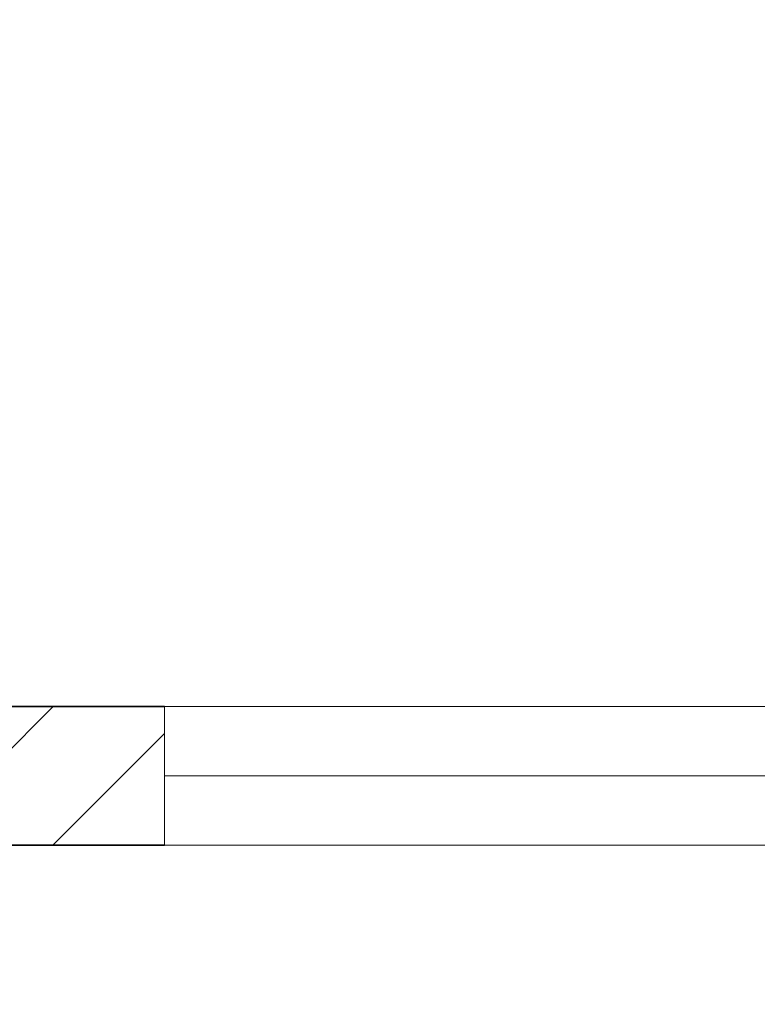
# Model space of a CAD drawing. Units: inches. Extents: x 1885 to 2748, y 783 to 2421.
# Tile 5 of 117: x 1993 to 2017, y 1082 to 1114. Entities that reach past the tile are written whole.
import ezdxf

# ---------------------------------------------------------------- set-up
doc = ezdxf.new("R2010")
doc.units = ezdxf.units.IN
doc.layers.add('A-GLAZ', color=181, linetype='Continuous', lineweight=18)
doc.layers.add('A-WALL', color=7, linetype='Continuous', lineweight=35)
doc.layers.add('A-WALL-PATT', color=85, linetype='Continuous', lineweight=13, true_color=0x58ba48)

# ---------------------------------------------------------------- blocks, each defined once
blk = doc.blocks.new('WIN-60')
for p, q in [((0.004, 59.998), (0.004, -0.002)), ((2.254, 59.998), (2.254, -0.002)), ((4.504, -0.002), (4.504, 59.998)), ((2.254, -0.002), (0.004, -0.002)), ((0.004, -0.002), (4.504, -0.002))]:
    blk.add_line(p, q)

msp = doc.modelspace()

# ---------------------------------------------------------------- hatches: boundary and pattern name
at = {"layer": 'A-WALL-PATT'}
h = msp.add_hatch(dxfattribs=at)
h.set_pattern_fill('ANSI32', color=256)
h.paths.add_polyline_path([(2007.772, 2318.006), (1980.774, 2318.006), (1980.774, 2281.215), (1985.274, 2281.215), (1985.274, 2313.506), (2007.772, 2313.506), (2007.772, 2315.756)])
h.paths.add_polyline_path([(2094.324, 2318.006), (2067.772, 2318.006), (2067.772, 2313.506), (2094.324, 2313.506), (2094.324, 2315.756)])
h.paths.add_polyline_path([(2131.367, 2315.756), (2131.367, 2318.006), (2131.189, 2318.006), (2112.609, 2318.006), (2112.609, 2313.506), (2117.274, 2313.506), (2117.274, 2255.201), (2121.774, 2255.201), (2121.774, 2313.506), (2131.367, 2313.506)])
h.paths.add_polyline_path([(2190.512, 2318.006), (2155.367, 2318.006), (2155.367, 2313.506), (2169.774, 2313.506), (2169.774, 2229.506), (2121.774, 2229.506), (2121.774, 2233.451), (2119.524, 2233.451), (2117.274, 2233.451), (2117.274, 2201.101), (2121.774, 2201.101), (2121.774, 2225.006), (2169.774, 2225.006), (2169.774, 2165.006), (2306.274, 2165.006), (2306.274, 2066.006), (2310.774, 2066.006), (2344.274, 2066.006), (2486.274, 2066.006), (2486.274, 1886.006), (2483.02, 1886.006), (2483.02, 1881.506), (2486.274, 1881.506), (2486.274, 1880.678), (2490.774, 1880.678), (2490.774, 2070.506), (2344.274, 2070.506), (2310.774, 2070.506), (2310.774, 2165.006), (2310.774, 2173.636), (2308.524, 2173.636), (2306.274, 2173.636), (2306.274, 2169.506), (2174.274, 2169.506), (2174.274, 2313.506), (2190.512, 2313.506), (2190.512, 2315.756)])
h.paths.add_polyline_path([(1985.274, 2221.215), (1980.774, 2221.215), (1980.774, 2165.006), (1992.774, 2165.006), (1992.774, 2141.927), (1997.274, 2141.927), (1997.274, 2165.006), (2117.274, 2165.006), (2117.274, 2163.126), (2121.774, 2163.126), (2121.774, 2172.734), (2119.524, 2172.734), (2117.274, 2172.734), (2117.274, 2169.506), (1985.274, 2169.506)])
h.paths.add_polyline_path([(1997.274, 2105.927), (1992.774, 2105.927), (1992.774, 2070.506), (2016.774, 2070.506), (2016.774, 2059.123), (2019.024, 2059.123), (2021.274, 2059.123), (2021.274, 2070.506), (2117.274, 2070.506), (2117.274, 2022.506), (2114.423, 2022.506), (2114.423, 2018.006), (2123.627, 2018.006), (2123.627, 2020.256), (2123.627, 2022.506), (2121.774, 2022.506), (2121.774, 2142.587), (2119.524, 2142.587), (2117.274, 2142.587), (2117.274, 2075.006), (1997.274, 2075.006)])
h.paths.add_polyline_path([(2092.029, 2020.256), (2092.029, 2022.506), (2021.274, 2022.506), (2021.274, 2035.123), (2016.774, 2035.123), (2016.774, 2018.006), (2016.774, 1978.784), (2021.274, 1978.784), (2021.274, 2018.006), (2092.029, 2018.006)])
h.paths.add_polyline_path([(2260.938, 2022.506), (2153.105, 2022.506), (2153.105, 2020.256), (2153.105, 2018.006), (2155.274, 2018.006), (2155.274, 1886.006), (2107.629, 1886.006), (2107.629, 1881.506), (2182.911, 1881.506), (2182.911, 1883.756), (2182.911, 1886.006), (2159.774, 1886.006), (2159.774, 2018.006), (2260.938, 2018.006), (2260.938, 2020.256)])
h.paths.add_polyline_path([(2047.629, 1883.756), (2047.629, 1886.006), (2021.274, 1886.006), (2021.274, 1918.784), (2019.024, 1918.784), (2016.774, 1918.784), (2016.774, 1881.506), (2047.629, 1881.506)])
h.paths.add_polyline_path([(2306.361, 1883.756), (2306.361, 1886.006), (2296.274, 1886.006), (2296.274, 1982.006), (2316.535, 1982.006), (2316.535, 1984.256), (2316.535, 1986.506), (2296.274, 1986.506), (2296.274, 2022.506), (2289.276, 2022.506), (2289.276, 2018.006), (2291.774, 2018.006), (2291.774, 1886.006), (2242.911, 1886.006), (2242.911, 1881.506), (2306.361, 1881.506)], flags=17)
h.paths.add_polyline_path([(1985.274, 1843.006), (2021.6, 1843.006), (2021.534, 1845.441), (2021.477, 1847.506), (1980.774, 1847.506), (1980.774, 1809.446), (1985.274, 1809.446)])
h.paths.add_polyline_path([(2131.482, 1845.256), (2131.482, 1847.506), (2081.534, 1847.506), (2081.534, 1843.006), (2117.274, 1843.006), (2117.274, 1784.147), (2119.524, 1784.147), (2121.774, 1784.147), (2121.774, 1843.006), (2131.482, 1843.006)])
h.paths.add_polyline_path([(2203.886, 1847.506), (2155.482, 1847.506), (2155.482, 1843.006), (2169.774, 1843.006), (2169.774, 1759.006), (2121.774, 1759.006), (2121.774, 1761.457), (2117.274, 1761.457), (2117.274, 1730.429), (2121.774, 1730.429), (2121.774, 1754.506), (2177.421, 1754.506), (2177.421, 1756.756), (2177.421, 1759.006), (2174.274, 1759.006), (2174.274, 1843.006), (2203.886, 1843.006)])
h.paths.add_polyline_path([(2335.554, 1845.256), (2335.554, 1847.506), (2239.886, 1847.506), (2239.886, 1843.006), (2306.274, 1843.006), (2306.274, 1759.006), (2199.486, 1759.006), (2199.486, 1754.506), (2310.774, 1754.506), (2310.774, 1843.006), (2335.554, 1843.006)])
h.paths.add_polyline_path([(2348.774, 2022.506), (2344.274, 2022.506), (2344.274, 1986.506), (2341.681, 1986.506), (2341.681, 1982.006), (2344.274, 1982.006), (2344.274, 1886.006), (2330.361, 1886.006), (2330.361, 1881.506), (2361.627, 1881.506), (2361.627, 1883.756), (2361.627, 1886.006), (2348.774, 1886.006)], flags=17)
h.paths.add_polyline_path([(2283.251, 2315.756), (2283.251, 2318.006), (2238.512, 2318.006), (2238.512, 2313.506), (2283.251, 2313.506)], flags=17)
h.paths.add_polyline_path([(2363.274, 2348.006), (2388.677, 2348.006), (2388.677, 2350.256), (2388.677, 2352.506), (2358.774, 2352.506), (2358.774, 2348.006), (2358.774, 2318.006), (2344.481, 2318.006), (2344.481, 2313.506), (2358.774, 2313.506), (2358.774, 2229.506), (2310.774, 2229.506), (2310.774, 2231.952), (2306.274, 2231.952), (2306.274, 2205.611), (2310.774, 2205.611), (2310.774, 2225.006), (2358.774, 2225.006), (2358.774, 2211.506), (2452.329, 2211.506), (2452.329, 2213.756), (2452.329, 2216.006), (2363.274, 2216.006), (2363.274, 2318.006)])
h.paths.add_polyline_path([(2310.774, 2313.506), (2320.481, 2313.506), (2320.481, 2315.756), (2320.481, 2318.006), (2302.728, 2318.006), (2302.728, 2313.506), (2306.274, 2313.506), (2306.274, 2251.076), (2310.774, 2251.076)], flags=17)
h.paths.add_polyline_path([(2490.774, 2352.506), (2486.274, 2352.506), (2448.677, 2352.506), (2448.677, 2348.006), (2486.274, 2348.006), (2486.274, 2318.006), (2486.274, 2216.006), (2481.78, 2216.006), (2481.78, 2211.506), (2486.274, 2211.506), (2486.274, 2165.006), (2493.289, 2165.006), (2493.289, 2167.256), (2493.289, 2169.506), (2490.774, 2169.506), (2490.774, 2313.506), (2494.429, 2313.506), (2494.429, 2318.006), (2490.774, 2318.006)])
h.paths.add_polyline_path([(2534.653, 2318.006), (2515.691, 2318.006), (2515.691, 2313.506), (2534.653, 2313.506), (2534.653, 2315.756)])
h.paths.add_polyline_path([(2618.274, 2318.006), (2594.653, 2318.006), (2594.653, 2313.506), (2613.774, 2313.506), (2613.774, 2281.706), (2618.274, 2281.706)])
h.paths.add_polyline_path([(2618.274, 2221.706), (2613.774, 2221.706), (2613.774, 2169.506), (2554.019, 2169.506), (2554.019, 2165.006), (2613.774, 2165.006), (2613.774, 2152.878), (2618.274, 2152.878)])
h.paths.add_polyline_path([(2618.274, 2128.878), (2616.024, 2128.878), (2613.774, 2128.878), (2613.774, 2117.006), (2529.774, 2117.006), (2529.774, 2165.006), (2532.848, 2165.006), (2532.848, 2169.506), (2522.867, 2169.506), (2522.867, 2165.006), (2525.274, 2165.006), (2525.274, 2117.006), (2525.274, 2112.506), (2525.274, 2108.576), (2529.774, 2108.576), (2529.774, 2112.506), (2613.774, 2112.506), (2613.774, 2080.19), (2618.274, 2080.19)])
h.paths.add_polyline_path([(2618.274, 2044.19), (2616.024, 2044.19), (2613.774, 2044.19), (2613.774, 2015.506), (2529.774, 2015.506), (2529.774, 2088.582), (2527.524, 2088.582), (2525.274, 2088.582), (2525.274, 2011.006), (2613.774, 2011.006), (2613.774, 1956.755), (2618.274, 1956.755)])
h.paths.add_polyline_path([(2618.274, 1881.506), (2618.274, 1896.755), (2613.774, 1896.755), (2613.774, 1881.506), (2613.774, 1847.506), (2592.715, 1847.506), (2592.715, 1843.006), (2613.774, 1843.006), (2613.774, 1765.006), (2613.774, 1760.506), (2609.621, 1760.506), (2609.621, 1756.006), (2613.774, 1756.006), (2613.774, 1660.006), (2608.544, 1660.006), (2608.544, 1655.506), (2613.774, 1655.506), (2613.774, 1508.158), (2618.274, 1508.158)])
h.paths.add_polyline_path([(2565.774, 1843.006), (2568.997, 1843.006), (2568.997, 1847.506), (2490.774, 1847.506), (2490.774, 1849.7), (2488.524, 1849.7), (2486.274, 1849.7), (2486.274, 1847.506), (2477.274, 1847.506), (2477.274, 1838.506), (2477.274, 1821.493), (2486.274, 1821.493), (2486.274, 1838.506), (2561.274, 1838.506), (2561.274, 1765.006), (2486.274, 1765.006), (2486.274, 1786.157), (2477.274, 1786.157), (2477.274, 1765.006), (2477.274, 1756.006), (2486.274, 1756.006), (2565.774, 1756.006), (2585.621, 1756.006), (2585.621, 1758.256), (2585.621, 1760.506), (2565.774, 1760.506), (2565.774, 1765.006)])
h.paths.add_polyline_path([(2486.274, 1651.006), (2561.274, 1651.006), (2561.274, 1567.006), (2486.274, 1567.006), (2486.274, 1591.321), (2477.274, 1591.321), (2477.274, 1567.006), (2477.274, 1558.006), (2477.274, 1555.439), (2481.774, 1555.439), (2481.774, 1558.006), (2568.653, 1558.006), (2568.653, 1560.256), (2568.653, 1562.506), (2565.774, 1562.506), (2565.774, 1655.506), (2584.544, 1655.506), (2584.544, 1657.756), (2584.544, 1660.006), (2565.774, 1660.006), (2486.274, 1660.006), (2477.274, 1660.006), (2477.274, 1651.006), (2477.274, 1632.989), (2486.274, 1632.989)])
h.paths.add_polyline_path([(2449.967, 1883.756), (2449.967, 1886.006), (2421.627, 1886.006), (2421.627, 1881.506), (2449.967, 1881.506)], flags=17)
h.paths.add_polyline_path([(2447.274, 1847.506), (2395.554, 1847.506), (2395.554, 1843.006), (2442.774, 1843.006), (2442.774, 1809.27), (2447.274, 1809.27)])
h.paths.add_polyline_path([(1985.274, 1749.446), (1980.774, 1749.446), (1980.774, 1694.504), (1985.274, 1694.504), (1985.274, 1694.506), (1986.897, 1694.506), (1986.897, 1697.78), (1986.897, 1699.006), (1985.274, 1699.006)])
h.paths.add_polyline_path([(2152.774, 1699.006), (2121.774, 1699.006), (2121.774, 1703.668), (2119.524, 1703.668), (2117.274, 1703.668), (2117.274, 1699.006), (2009.219, 1699.006), (2009.219, 1694.506), (2148.274, 1694.506), (2148.274, 1692.631), (2152.774, 1692.631)])
h.paths.add_polyline_path([(2016.274, 1694.506), (2011.774, 1694.506), (2011.774, 1558.006), (2040.806, 1558.006), (2040.806, 1560.256), (2040.806, 1562.506), (2016.274, 1562.506)])
h.paths.add_polyline_path([(2152.774, 1663.017), (2150.524, 1663.017), (2148.274, 1663.017), (2148.274, 1562.506), (2100.806, 1562.506), (2100.806, 1558.006), (2165.119, 1558.006), (2165.119, 1560.256), (2165.119, 1562.506), (2152.774, 1562.506), (2152.774, 1610.506), (2224.774, 1610.506), (2224.774, 1607.99), (2229.274, 1607.99), (2229.274, 1615.006), (2152.774, 1615.006)])
h.paths.add_polyline_path([(2238.613, 1560.256), (2238.613, 1562.506), (2229.274, 1562.506), (2229.274, 1588.756), (2227.024, 1588.763), (2224.774, 1588.771), (2224.774, 1562.506), (2189.119, 1562.506), (2189.119, 1558.006), (2238.613, 1558.006)])
h.paths.add_polyline_path([(2336.024, 1560.256), (2336.024, 1562.506), (2310.774, 1562.506), (2310.774, 1656.347), (2308.524, 1656.347), (2306.274, 1656.347), (2306.274, 1562.506), (2286.613, 1562.506), (2286.613, 1558.006), (2336.024, 1558.006)])
h.paths.add_polyline_path([(2447.274, 1690.968), (2445.024, 1690.968), (2442.774, 1690.968), (2442.774, 1687.006), (2306.274, 1687.006), (2306.274, 1680.75), (2310.774, 1680.75), (2310.774, 1682.506), (2442.774, 1682.506), (2442.774, 1562.506), (2396.024, 1562.506), (2396.024, 1558.006), (2447.274, 1558.006)])
h.paths.add_polyline_path([(2447.274, 1749.27), (2445.024, 1749.27), (2442.774, 1749.27), (2442.774, 1717.232), (2447.274, 1717.232)])
h.paths.add_polyline_path([(2044.674, 1521.756), (2044.674, 1524.006), (2007.274, 1524.006), (2007.274, 1503.49), (2009.524, 1503.49), (2011.774, 1503.49), (2011.774, 1519.506), (2044.674, 1519.506)])
h.paths.add_polyline_path([(2177.969, 1521.756), (2177.969, 1524.006), (2104.674, 1524.006), (2104.674, 1519.506), (2145.774, 1519.506), (2145.774, 1387.506), (2143.37, 1387.506), (2143.37, 1383.006), (2251.585, 1383.006), (2251.585, 1385.256), (2251.585, 1387.506), (2150.274, 1387.506), (2150.274, 1519.506), (2177.969, 1519.506)])
h.paths.add_polyline_path([(2298.704, 1524.006), (2237.969, 1524.006), (2237.969, 1519.506), (2282.274, 1519.506), (2282.274, 1387.506), (2279.683, 1387.506), (2279.683, 1383.006), (2286.774, 1383.006), (2286.774, 1419.006), (2312.451, 1419.006), (2312.451, 1421.256), (2312.451, 1423.506), (2286.774, 1423.506), (2286.774, 1519.506), (2298.704, 1519.506), (2298.704, 1521.722)], flags=17)
h.paths.add_polyline_path([(2361.897, 1521.756), (2361.897, 1524.006), (2322.704, 1524.006), (2322.704, 1519.506), (2334.774, 1519.506), (2334.774, 1423.506), (2331.93, 1423.506), (2331.93, 1419.006), (2334.774, 1419.006), (2334.774, 1387.506), (2334.774, 1383.228), (2339.274, 1383.228), (2339.274, 1387.506), (2339.274, 1519.506), (2361.897, 1519.506)], flags=17)
h.paths.add_polyline_path([(2447.274, 1521.756), (2447.274, 1524.006), (2421.897, 1524.006), (2421.897, 1519.506), (2447.274, 1519.506)], flags=17)
h.paths.add_polyline_path([(2481.774, 1529.6), (2479.524, 1529.6), (2477.274, 1529.6), (2477.274, 1524.006), (2474.489, 1524.006), (2474.489, 1519.506), (2477.274, 1519.506), (2477.274, 1334.506), (2296.774, 1334.506), (2296.774, 1240.506), (2160.274, 1240.506), (2160.274, 1180.506), (2112.274, 1180.506), (2112.274, 1207.692), (2110.024, 1207.692), (2107.774, 1207.692), (2107.774, 1171.609), (2112.274, 1171.609), (2112.274, 1176.006), (2160.274, 1176.006), (2160.274, 1092.006), (2144.221, 1092.006), (2144.221, 1087.506), (2189.497, 1087.506), (2189.497, 1089.756), (2189.497, 1092.006), (2164.774, 1092.006), (2164.774, 1236.006), (2296.774, 1236.006), (2296.774, 1231.912), (2301.274, 1231.912), (2301.274, 1330.006), (2481.774, 1330.006), (2481.774, 1387.506)])
h.paths.add_polyline_path([(2618.274, 1448.158), (2613.774, 1448.158), (2613.774, 1382.506), (2529.774, 1382.506), (2525.274, 1382.506), (2525.274, 1307.062), (2529.774, 1307.062), (2529.774, 1378.006), (2613.774, 1378.006), (2613.774, 1354.988), (2618.274, 1354.988)])
h.paths.add_polyline_path([(2618.274, 1318.988), (2613.774, 1318.988), (2613.774, 1281.006), (2529.774, 1281.006), (2529.774, 1283.786), (2527.524, 1283.786), (2525.274, 1283.786), (2525.274, 1228.506), (2516.794, 1228.506), (2516.794, 1224.006), (2533.484, 1224.006), (2533.484, 1226.256), (2533.484, 1228.506), (2529.774, 1228.506), (2529.774, 1276.506), (2613.774, 1276.506), (2613.774, 1266.02), (2618.274, 1266.02)])
h.paths.add_polyline_path([(2618.274, 1134.964), (2613.774, 1134.964), (2613.774, 1092.006), (2594.545, 1092.006), (2594.545, 1087.506), (2618.274, 1087.506)])
h.paths.add_polyline_path([(2534.545, 1092.006), (2509.765, 1092.006), (2509.765, 1087.506), (2534.545, 1087.506), (2534.545, 1089.756)])
h.paths.add_polyline_path([(2481.274, 1224.006), (2484.117, 1224.006), (2484.117, 1226.256), (2484.117, 1228.506), (2476.774, 1228.506), (2476.774, 1198.506), (2471.61, 1198.506), (2471.61, 1194.006), (2476.774, 1194.006), (2476.774, 1062.006), (2436.894, 1062.006), (2436.894, 1057.506), (2476.774, 1057.506), (2481.274, 1057.506), (2481.274, 1062.006), (2481.274, 1087.506), (2485.354, 1087.506), (2485.354, 1089.756), (2485.354, 1092.006), (2481.274, 1092.006), (2481.274, 1117.506)])
h.paths.add_polyline_path([(2439.898, 1198.506), (2349.274, 1198.506), (2349.274, 1194.006), (2349.274, 1180.506), (2301.274, 1180.506), (2301.274, 1201.896), (2299.024, 1201.896), (2296.774, 1201.896), (2296.774, 1172.335), (2299.024, 1172.335), (2301.274, 1172.335), (2301.274, 1176.006), (2349.274, 1176.006), (2349.274, 1092.006), (2334.452, 1092.006), (2334.452, 1087.506), (2349.274, 1087.506), (2349.274, 1057.506), (2353.774, 1057.506), (2376.894, 1057.506), (2376.894, 1059.756), (2376.894, 1062.006), (2353.774, 1062.006), (2353.774, 1087.506), (2353.774, 1180.506), (2353.774, 1194.006), (2439.898, 1194.006), (2439.898, 1196.256)])
h.paths.add_polyline_path([(2270.596, 1089.756), (2270.596, 1092.006), (2249.497, 1092.006), (2249.497, 1087.506), (2270.596, 1087.506)], flags=17)
h.paths.add_polyline_path([(2310.452, 1092.006), (2301.274, 1092.006), (2301.274, 1153.292), (2296.774, 1153.292), (2296.774, 1092.006), (2293.786, 1092.006), (2293.786, 1087.506), (2310.452, 1087.506), (2310.452, 1089.756)], flags=17)
h.paths.add_polyline_path([(2112.274, 1150.328), (2110.024, 1150.328), (2107.774, 1150.328), (2107.774, 1092.006), (2104.465, 1092.006), (2104.465, 1087.506), (2120.221, 1087.506), (2120.221, 1089.756), (2120.221, 1092.006), (2112.274, 1092.006)])
h.paths.add_polyline_path([(2082.172, 1092.006), (2058.144, 1092.006), (2058.144, 1087.506), (2082.172, 1087.506), (2082.172, 1089.756)])
h.paths.add_polyline_path([(1975.774, 1145.638), (1971.274, 1145.638), (1971.274, 1087.506), (1980.774, 1087.506), (1998.144, 1087.506), (1998.144, 1089.756), (1998.144, 1092.006), (1985.274, 1092.006), (1975.774, 1092.006)])
h.paths.add_polyline_path([(2112.274, 1244.385), (2110.024, 1244.385), (2107.774, 1244.385), (2107.774, 1240.506), (1992.274, 1240.506), (1992.274, 1271.008), (1987.774, 1271.008), (1987.774, 1240.506), (1980.774, 1240.506), (1975.774, 1240.506), (1971.274, 1240.506), (1971.274, 1205.638), (1975.774, 1205.638), (1975.774, 1236.006), (2107.774, 1236.006), (2107.774, 1233.444), (2112.274, 1233.444), (2112.274, 1236.006)])
h.paths.add_polyline_path([(2112.274, 1383.006), (2114.783, 1383.006), (2114.783, 1385.256), (2114.783, 1387.506), (2102.476, 1387.506), (2102.476, 1383.006), (2107.774, 1383.006), (2107.774, 1335.006), (2011.774, 1335.006), (2011.774, 1349.939), (2007.274, 1349.939), (2007.274, 1335.006), (1987.774, 1335.006), (1987.774, 1330.506), (1987.774, 1307.008), (1992.274, 1307.008), (1992.274, 1330.506), (2007.274, 1330.506), (2107.774, 1330.506), (2107.774, 1264.711), (2112.274, 1264.711)])
h.paths.add_polyline_path([(2077.857, 1387.506), (2011.774, 1387.506), (2011.774, 1390.036), (2009.524, 1390.036), (2007.274, 1390.036), (2007.274, 1373.939), (2011.774, 1373.939), (2011.774, 1383.006), (2077.857, 1383.006)])
h.paths.add_polyline_path([(2011.774, 1443.49), (2007.274, 1443.49), (2007.274, 1410.248), (2011.774, 1410.248)])

# ---------------------------------------------------------------- linework, layer by layer
at = {"layer": 'A-WALL'}
for p, q in [((1998.144, 1092.006), (1985.274, 1092.006)), ((1998.144, 1087.506), (1980.774, 1087.506))]:
    msp.add_line(p, q, dxfattribs=at)

# ---------------------------------------------------------------- block references
at = {"layer": 'A-GLAZ', "extrusion": (0, 0, -1), "zscale": -1, "rotation": 90}
msp.add_blockref('WIN-60', (-1998.146, 1087.502), dxfattribs=at)

doc.saveas('drawing.dxf')
